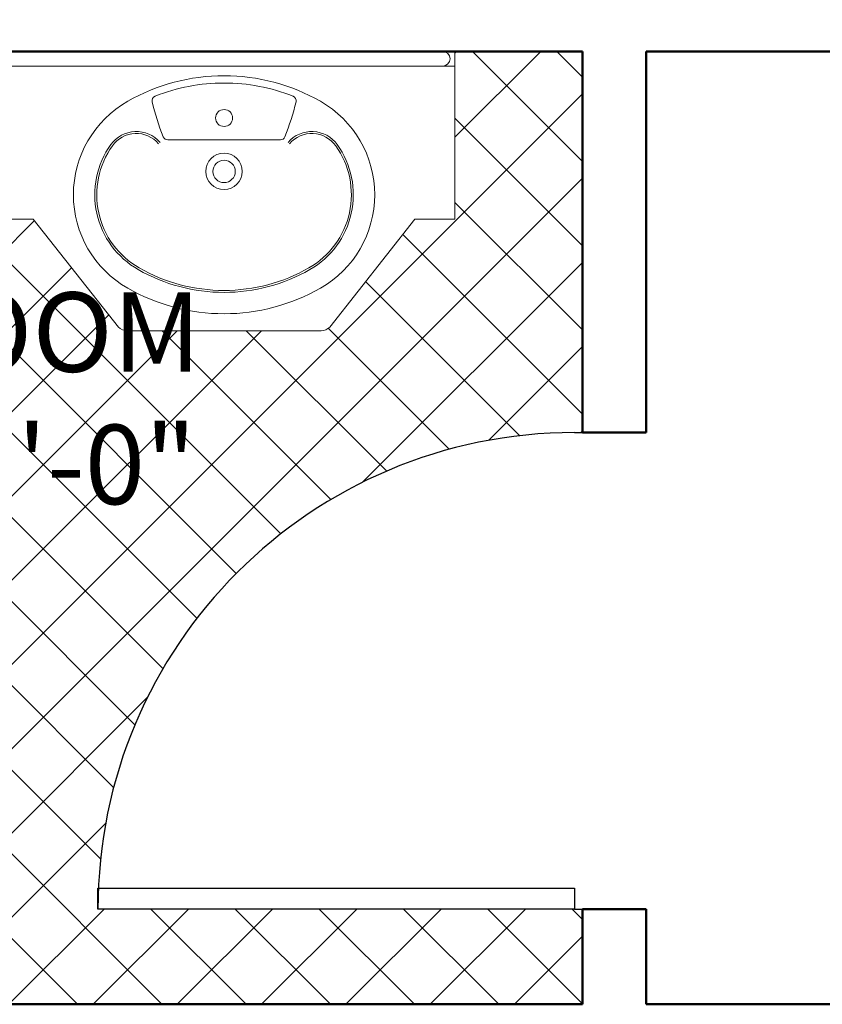
# Model space of a CAD drawing. Units: inches. Extents: x -466983 to 1020, y 324 to 318697.
# Tile 5 of 97: x 504 to 555, y 567 to 629. Entities that reach past the tile are written whole.
import ezdxf

# ---------------------------------------------------------------- set-up
doc = ezdxf.new("R2010")
doc.units = ezdxf.units.IN
doc.header["$MEASUREMENT"] = 0
for name, color, linetype, lineweight in [('A-AREA-IDEN', 7, 'Continuous', 25), ('A-DOOR', 3, 'Continuous', 25), ('A-FLOR-FIXT', 9, 'Continuous', 18), ('A-FLOR-PATT', 252, 'Continuous', 13), ('A-WALL', 7, 'Continuous', 50)]:
    doc.layers.add(name, color=color, linetype=linetype, lineweight=lineweight)
doc.styles.get("Standard").update_dxf_attribs({"font": 'arial.ttf'})

# ---------------------------------------------------------------- blocks, each defined once
blk = doc.blocks.new('*U33')
for p, q in [((0, 0), (-1e-16, -5.999999999999999)), ((40, -6e-16), (40, -6))]:
    blk.add_line(p, q)
blk.add_lwpolyline([(0, 0), (5.6e-15, 40), (1.750000000000007, 40), (1.749999999999998, -7e-16)], close=True)
blk.add_arc((0, 0), 40, 0, 90)
blk = doc.blocks.new('B3')
for p, q in [((-450, 0), (-455.7402514854766, -1.1418070123309)), ((450, 0), (455.7402514854766, -1.1418070123309)), ((-463.8581929876745, -9.25974851452338), (-465, -15)), ((-465, -15), (-463.8581929876745, -20.74025148547662)), ((-460.6066017178018, -4.393398282201815), (-463.8581929876745, -9.25974851452338)), ((-455.7402514854766, -1.1418070123309), (-460.6066017178018, -4.393398282201815)), ((455.7402514854766, -1.1418070123309), (460.6066017177945, -4.393398282201815)), ((460.6066017177945, -4.393398282201815), (463.8581929876672, -9.25974851452338)), ((463.8581929876672, -9.25974851452338), (465, -15)), ((465, -15), (463.8581929876672, -20.74025148547662)), ((475, -30), (-475, -30)), ((-463.8581929876745, -20.74025148547662), (-460.6066017178018, -25.60660171779819)), ((-460.6066017178018, -25.60660171779819), (-455.7402514854766, -28.8581929876691)), ((-455.7402514854766, -28.8581929876691), (-450, -30)), ((455.7402514854766, -28.8581929876691), (450, -30)), ((460.6066017177945, -25.60660171779819), (455.7402514854766, -28.8581929876691)), ((463.8581929876672, -20.74025148547662), (460.6066017177945, -25.60660171779819)), ((2.91038e-11, -182.0000000000054), (-115.8117069986983, -182.0000000000054)), ((2.91038e-11, -182.0000000000054), (115.8117069987565, -182.0000000000054))]:
    blk.add_line(p, q)
blk.add_lwpolyline([(199.4833683843535, -575, 0.2017697719241106), (217.3542190239823, -567.482353886593), (392.5, -345), (435, -345), (475, -345), (475, 0), (-475, 0), (-475, -345), (-435, -345), (-392.5, -345), (-217.3542190239896, -567.482353886593, 0.2017697719241107), (-199.4833683843608, -575)], format="xyb", close=True)
for centre, radius, start, end in [((5.09317e-11, -450.0000000000327), 400.0000000000322, 90, 119.7172288959075), ((0, -450.0000000000327), 400.0000000000319, 60.28277110409252, 90), ((2.91038e-11, -450.0000000000055), 385, 90, 111.6513567404431), ((2.91038e-11, -450.0000000000055), 385, 68.34864325955687, 90), ((-138.3591766736499, -101.4576952073475), 10, 111.6513567404431, 193.3915177581575), ((138.3591766737008, -101.4576952073475), 10, 346.6084822418425, 68.34864325955687), ((-88.47222222221171, -295.0000000000055), 221.527777777762, 119.7172288959075, 240.2827711040925), ((338.3178096717893, 12.0282100348104), 500, 193.3915177581575, 202.0594091764406), ((2.91038e-11, -136.9999999999891), 17.5, 90, 270), ((2.91038e-11, -136.9999999999891), 17.5, 270, 90), ((-338.3178096717383, 12.0282100348104), 500, 337.9405908235594, 346.6084822418425), ((88.47222222225537, -294.9999999999964), 221.527777777762, 299.7172288959074, 60.28277110409252), ((-180.5137974189128, -229.2550553338115), 64.41699441097052, 40.71477974361456, 144.4619255202982), ((-180.5137974189128, -229.2550553338115), 60.41699441097051, 40.71477974361456, 144.4619255202982), ((-115.8117069986983, -172.0000000000145), 10, 202.0594091764406, 270), ((115.8117069987565, -172.0000000000145), 10, 270, 337.9405908235594), ((180.5137974189638, -229.2550553338115), 64.41699441097052, 35.53807447970174, 139.2852202563854), ((180.5137974189638, -229.2550553338115), 60.41699441097051, 35.53807447970174, 139.2852202563854), ((-88.47222222221171, -295.0000000000055), 177.5277777777778, 144.4619255202982, 240.2827711040925), ((-88.47222222221171, -295.0000000000055), 173.5277777777778, 144.4619255202982, 240.2827711040925), ((88.47222222223354, -295.0000000000055), 173.5277777777778, 299.7172288959074, 35.53807447970174), ((88.47222222223354, -295.0000000000055), 177.5277777777778, 299.7172288959074, 35.53807447970174), ((2.91038e-11, -247.0000000000037), 37.5, 90, 270), ((2.91038e-11, -247.0000000000037), 37.5, 270, 90), ((2.91038e-11, -247.0000000000037), 23, 90, 270), ((2.91038e-11, -247.0000000000037), 23, 270, 90), ((2.91038e-11, -140.0000000000036), 352, 240.2827711040925, 270), ((2.91038e-11, -140.0000000000036), 352, 270, 299.7172288959074), ((2.91038e-11, -140.0000000000036), 356, 240.2827711040925, 270), ((2.91038e-11, -140.0000000000036), 356, 270, 299.7172288959074), ((5.09317e-11, -139.9999999999781), 400.0000000000309, 240.2827711040925, 270), ((-1.45519e-11, -140.0000000000309), 399.9999999999781, 270, 299.7172288959074)]:
    blk.add_arc(centre, radius, start, end)

msp = doc.modelspace()

# ---------------------------------------------------------------- hatches: boundary and pattern name
at = {"layer": 'A-FLOR-PATT', "transparency": 33554572}
h = msp.add_hatch(dxfattribs=at)
h.set_pattern_fill('ANSI37', color=256, scale=30)
h.set_pattern_definition([(45, (-1212.413693079869, -290.0350025265127), (-2.651650429449553, 2.651650429449553), []), (135, (-1212.413693079869, -290.0350025265127), (-2.651650429449553, -2.651650429449552), [])])
h.paths.add_polyline_path([(901.805677520904, 1075.937732818422), (900.6144036774049, 1075.937732818422), (900.6144036774049, 1065.385628316983), (899.390971271441, 1065.385628316983), (898.0910743401043, 1065.385628316983), (892.8355944880973, 1058.709752245277, -0.2583770168556315), (892.18750428989, 1058.350891982691), (879.9847834232776, 1058.350891982691, -0.2017697719240963), (879.438188978411, 1058.580825279484), (874.0812133730635, 1065.385628316983), (872.7813164417267, 1065.385628316983), (871.5578840357629, 1065.385628316983), (871.5578840357629, 1075.937732818422), (813.8056775209042, 1075.937732818422), (813.8056775209042, 1044.792233318721), (832.3947444543938, 1044.792233318721, -0.3947951267487684), (848.6601780212009, 1028.535584015862), (848.6601780212009, 1009.937732818421), (901.805677520904, 1009.937732818421), (901.805677520904, 1015.937732818421), (901.3056775209042, 1015.937732818421), (871.3056775209039, 1015.937732818421), (871.3056775209039, 1017.250232818421), (871.3344022102003, 1017.250232818421, -0.4014527144963572), (901.3056775209042, 1045.937732818421), (901.805677520904, 1045.937732818421)])
edge = h.paths.add_edge_path(flags=16)
edge.add_line((847.7730719745084, 1068.948588737025), (847.7730719745069, 1073.708823774771))
edge.add_arc((849.2268986539951, 1073.708823774771), 1.453826679487974, 90, 180, ccw=False)
edge.add_line((849.2268986539951, 1075.162650454259), (864.4920787886183, 1075.162650454259))
edge.add_arc((864.4920787886213, 1073.708823774771), 1.453826679487974, 0, 90.00000000012102, ccw=False)
edge.add_line((865.9459054681093, 1073.708823774771), (865.9459054681081, 1069.00351244647))
edge.add_arc((832.6447385074767, 1068.976050591752), 33.30117828385809, -20.61233806670998, 0.04724903539101888, ccw=False)
edge.add_ellipse((856.8594887213083, 1058.479989307073), major_axis=(-2.091e-13, 10.21313242340307), ratio=0.6859192225533502, start_angle=100.00884331843292, end_angle=259.9911566815624, ccw=False)
edge.add_arc((881.0742389351396, 1068.976050591752), 33.30117828385809, 180.0472490354062, 200.6123380667097, ccw=False)
h.paths.add_polyline_path([(853.145578187156, 1066.481532374271), (853.145578187156, 1066.453444752512), (853.1463399851561, 1066.453444752512, 0.4331071439582673), (852.9166149812349, 1066.684892837266), (852.9166149812349, 1066.453444752512), (853.145578187156, 1066.453444752512), (853.145578187156, 1066.481532374489), (853.088019486549, 1066.612171966583, 0.6979386910037918), (852.699540939094, 1066.453444752512), (852.7003027371272, 1066.453444752512), (852.7003027371272, 1066.481532374489), (852.9166149812349, 1067.001204630995), (852.9166149812349, 1066.684892837266, -0.3962543063594317)], flags=0)
h.paths.add_polyline_path([(861.0186747055222, 1066.481532374271), (861.0186747055222, 1066.453444752512), (861.0194365035225, 1066.453444752512, 0.4164039232557909), (860.8023624614146, 1066.684892837265), (860.8023624614146, 1066.453444752512), (861.0186747055222, 1066.453444752512), (861.0186747055222, 1066.481532374489), (860.9671752720659, 1066.605255499379, 0.7133437187663149), (860.5726374574602, 1066.453444752512), (860.5733992554934, 1066.453444752512), (860.5733992554934, 1066.481532374489), (860.8023624614146, 1067.001204630995), (860.8023624614146, 1066.684892837265, -0.3799725304814568)], flags=0)
edge = h.paths.add_edge_path(flags=0)
edge.add_spline(control_points=[(861.1298377106021, 1065.785468371534), (861.4660965533383, 1065.247811229462), (861.613385559155, 1065.016139861057), (861.9832837951076, 1064.373617117607), (862.1924105327118, 1063.944313665492), (862.5613774174725, 1063.039129539609), (862.7212131906668, 1062.56326642291), (862.9865156700853, 1061.578122280975), (863.0919804897928, 1061.068856600952), (863.2452407883674, 1060.031049745086), (863.293035446714, 1059.502522766744), (863.3294736797056, 1058.440879580113), (863.3181170778639, 1057.907777155726), (863.2366033468288, 1056.85179603536), (863.1664466211855, 1056.328931215311), (862.9695120306455, 1055.307951977375), (862.8427353108815, 1054.809852090196), (862.5365466723708, 1053.852219447362), (862.3571373353129, 1053.392702749349), (861.9514237071658, 1052.524888245794), (861.7251255454219, 1052.116609101398), (861.2330086320977, 1051.362239687588), (860.9672044472572, 1051.016170456457), (860.4047960485765, 1050.394909316517), (860.1082220871676, 1050.119734477926), (859.493696255806, 1049.64606200509), (859.1757900615103, 1049.447558762665), (858.5275631429041, 1049.129883644436), (858.197273503909, 1049.010664382187), (857.5314773710529, 1048.851811036626), (857.1959384637446, 1048.812116564677), (856.5249326641573, 1048.811967422545), (856.1893892160524, 1048.851512676201), (855.5235728169741, 1049.010066967686), (855.1932673158994, 1049.129136347874), (854.5449932971788, 1049.446513839261), (854.2270557868354, 1049.644869411481), (853.6124495619564, 1050.118254324803), (853.3158265363004, 1050.393289340464), (852.7533025914207, 1051.014284587242), (852.487431959371, 1051.360227769297), (851.9951668313728, 1052.114363776776), (851.7687869247744, 1052.522535562859), (851.3628973914427, 1053.390157753425), (851.1833939042357, 1053.849589492002), (850.8770077813263, 1054.807077270704), (850.7501277313783, 1055.30511724975), (850.5529806633081, 1056.326003473117), (850.4827147921034, 1056.848835185142), (850.4009803807432, 1057.904777820697), (850.3895122452288, 1058.437874867502), (850.425728471152, 1059.499535178563), (850.4734126571939, 1060.02808465918), (850.6264565107679, 1061.065963770327), (850.7318153592672, 1061.575279204679), (850.9969137893603, 1062.560548677974), (851.1566514873134, 1063.036487374614), (851.525433403113, 1063.94184619004), (851.7344732542367, 1064.371248757046), (852.1056260411488, 1065.016350037675), (852.2544071072941, 1065.250281998093), (852.608154630964, 1065.733465727338)], knot_values=[3.915332106759953, 3.915332106759953, 3.915332106759953, 3.915332106759953, 4.013467662305501, 4.013467662305501, 4.175531746215815, 4.175531746215815, 4.337595830126129, 4.337595830126129, 4.499659914036444, 4.499659914036444, 4.661723997946757, 4.661723997946757, 4.82378808185707, 4.82378808185707, 4.985852165767384, 4.985852165767384, 5.147916249677697, 5.147916249677697, 5.30998033358801, 5.30998033358801, 5.472044417498324, 5.472044417498324, 5.634108501408637, 5.634108501408637, 5.79617258531895, 5.79617258531895, 5.958236669229264, 5.958236669229264, 6.120300753139577, 6.120300753139577, 6.282364837049891, 6.282364837049891, 6.444428920960204, 6.444428920960204, 6.606493004870517, 6.606493004870517, 6.768557088780831, 6.768557088780831, 6.930621172691144, 6.930621172691144, 7.092685256601457, 7.092685256601457, 7.254749340511771, 7.254749340511771, 7.416813424422084, 7.416813424422084, 7.578877508332397, 7.578877508332397, 7.740941592242711, 7.740941592242711, 7.903005676153024, 7.903005676153024, 8.065069760063338, 8.065069760063338, 8.22713384397365, 8.22713384397365, 8.389197927883965, 8.389197927883965, 8.551262011794279, 8.551262011794279, 8.650370494357087, 8.650370494357087, 8.650370494357087, 8.650370494357087], degree=3, periodic=0)
edge.add_line((852.6421178657537, 1065.785468371534), (861.1298377106024, 1065.785468371534))
edge = h.paths.add_edge_path(flags=0)
edge.add_ellipse((856.8495804607978, 1057.743205248224), major_axis=(-3.1e-13, 7.792134415209829), ratio=0.6878610933899516, start_angle=0, end_angle=360)
h.paths.add_polyline_path([(848.8634419841151, 1069.389059844444), (848.863441984139, 1073.960453158315, -0.4142135623709757), (849.9538119937549, 1075.050823167924), (863.765165448898, 1075.050823167924, -0.4142135623721942), (864.8555354585106, 1073.960453158308), (864.8555354584933, 1069.389059844444, -0.3889362887010341), (864.5236837164459, 1069.026979909221, -0.0435607626104464), (849.19529372618, 1069.02697990933, -0.3889362886276668)], flags=0)
h.paths.add_polyline_path([(853.1006153779753, 1068.112209480768, -1), (852.677499999749, 1068.112209480768, -1)], flags=0)
edge = h.paths.add_edge_path(flags=0)
edge.add_ellipse((856.8594887213083, 1057.33782914961), major_axis=(7.74e-14, 2.20702192546696), ratio=0.6571642650458812, start_angle=0, end_angle=360)
h.paths.add_polyline_path([(861.0414774428674, 1068.112209480768, -1), (860.6183620646412, 1068.112209480768, -1)], flags=0)
edge = h.paths.add_edge_path()
edge.add_line((573.9536545579417, 1057.341203598636), (573.9536545579417, 1075.937732818422))
edge.add_line((573.9536545579417, 1075.937732818422), (558.7307922536265, 1075.937732818422))
edge.add_line((558.7307922536265, 1075.937732818422), (558.7307922536265, 1065.385628316983))
edge.add_line((558.7307922536265, 1065.385628316983), (557.5073598476627, 1065.385628316983))
edge.add_line((557.5073598476627, 1065.385628316983), (556.207462916326, 1065.385628316983))
edge.add_line((556.207462916326, 1065.385628316983), (550.9519830643189, 1058.709752245277))
edge.add_arc((550.3038928661116, 1059.115537236419), 0.7646452537275144, 270, 327.94831933647396, ccw=False)
edge.add_line((550.3038928661116, 1058.350891982691), (538.1011719994992, 1058.350891982691))
edge.add_arc((538.1011719994992, 1059.115537236419), 0.7646452537275137, 224.3704013916024, 270, ccw=False)
edge.add_line((537.5545775546327, 1058.580825279484), (532.1976019492852, 1065.385628316983))
edge.add_line((532.1976019492852, 1065.385628316983), (530.8977050179485, 1065.385628316983))
edge.add_line((530.8977050179485, 1065.385628316983), (529.6742726119846, 1065.385628316983))
edge.add_line((529.6742726119846, 1065.385628316983), (529.6742726119846, 1075.937732818422))
edge.add_line((529.6742726119846, 1075.937732818422), (520.8056775209042, 1075.937732818422))
edge.add_line((520.8056775209042, 1075.937732818422), (520.8056775209042, 1045.937732818422))
edge.add_line((520.8056775209042, 1045.937732818422), (521.3056775209044, 1045.937732818422))
edge.add_arc((521.3056775209042, 1015.937732818422), 30.00000000000023, 2.507490703587223, 89.99999999999977, ccw=False)
edge.add_line((551.2769528316082, 1017.250232818422), (551.3056775209045, 1017.250232818422))
edge.add_line((551.3056775209045, 1017.250232818422), (551.3056775209045, 1015.937732818422))
edge.add_line((551.3056775209045, 1015.937732818422), (520.8056775209042, 1015.937732818422))
edge.add_line((520.8056775209042, 1015.937732818422), (520.8056775209042, 1009.937732818421))
edge.add_line((520.8056775209042, 1009.937732818421), (559.1912990237018, 1010.402158339383))
edge.add_arc((559.1912990237018, 1011.855985018871), 1.453826679487974, 180, 270, ccw=False)
edge.add_line((557.7374723442138, 1011.855985018871), (557.7374723442151, 1016.561296347171))
edge.add_arc((591.0386393048469, 1016.58875820189), 33.3011782838587, 159.3876619332891, 180.0472490353913, ccw=False)
edge.add_ellipse((566.8238890910148, 1027.084819486569), major_axis=(-3.171e-13, 10.21313242340307), ratio=0.6859192225533445, start_angle=280.00884331843395, end_angle=439.99115668156304, ccw=False)
edge.add_arc((542.6091388771833, 1016.58875820189), 33.3011782838584, 0.04724903544490644, 20.612338066710322, ccw=False)
edge.add_line((575.9103058378148, 1016.61622005664), (575.910305837816, 1011.855985018871))
edge.add_arc((574.4564791583282, 1011.855985018871), 1.453826679487974, -90, 0, ccw=False)
edge.add_line((574.4564791583282, 1010.402158339383), (608.8056775209044, 1009.937732818421))
edge.add_line((608.8056775209044, 1009.937732818421), (608.8056775209044, 1041.08570985546))
edge.add_line((608.8056775209044, 1041.08570985546), (590.2179319406538, 1041.08570985546))
edge.add_arc((590.7750219589672, 1057.907380652626), 16.83089295601249, 181.9277454211679, 268.1032059320871, ccw=False)
edge = h.paths.add_edge_path()
edge.add_ellipse((494.2443328575609, 583.6203939656394), major_axis=(-2.099e-13, 10.21313242340307), ratio=0.6859192225533391, start_angle=280.0088433184392, end_angle=439.99115668155895, ccw=False)
edge.add_arc((470.0295826437295, 573.1243326809605), 33.30117828385828, 0.047249035653180727, 20.612338066711573, ccw=False)
edge.add_line((503.3307496043607, 573.1517945358311), (503.3307496043621, 568.3915594979414))
edge.add_arc((501.8769229248741, 568.3915594979414), 1.453826679487974, -90, 0, ccw=False)
edge.add_line((501.8769229248741, 566.9377328184536), (539.8056775209043, 566.9377328184218))
edge.add_line((539.8056775209043, 566.9377328184218), (539.8056775209043, 572.9377328184218))
edge.add_line((539.8056775209043, 572.9377328184218), (539.3056775209043, 572.9377328184218))
edge.add_line((539.3056775209043, 572.9377328184218), (509.3056775209042, 572.9377328184218))
edge.add_line((509.3056775209042, 572.9377328184218), (509.3056775209042, 574.2502328184218))
edge.add_line((509.3056775209042, 574.2502328184218), (509.3344022102004, 574.2502328184218))
edge.add_arc((539.3056775209043, 572.9377328184218), 30.00000000000003, 90, 177.4925092964128, ccw=False)
edge.add_line((539.3056775209043, 602.9377328184218), (539.8056775209043, 602.9377328184218))
edge.add_line((539.8056775209043, 602.9377328184218), (539.8056775209043, 626.9377328184219))
edge.add_line((539.8056775209043, 626.9377328184219), (531.7718318056131, 626.9377328184219))
edge.add_line((531.7718318056131, 626.9377328184219), (531.7718318056131, 616.3856283169836))
edge.add_line((531.7718318056131, 616.3856283169836), (530.5483993996492, 616.3856283169836))
edge.add_line((530.5483993996492, 616.3856283169836), (529.2485024683125, 616.3856283169836))
edge.add_line((529.2485024683125, 616.3856283169836), (523.7105154427977, 609.3508919826913))
edge.add_line((523.7105154427977, 609.3508919826913), (510.7766285267865, 609.3508919826913))
edge.add_line((510.7766285267865, 609.3508919826913), (505.2386415012717, 616.3856283169835))
edge.add_line((505.2386415012717, 616.3856283169835), (503.9387445699351, 616.3856283169836))
edge.add_line((503.9387445699351, 616.3856283169836), (502.7153121639711, 616.3856283169836))
edge.add_line((502.7153121639711, 616.3856283169836), (502.7153121639712, 626.9377328184219))
edge.add_line((502.7153121639712, 626.9377328184219), (481.698294634846, 626.937732818422))
edge.add_line((481.698294634846, 626.937732818422), (481.6982946348461, 610.9950036909872))
edge.add_arc((467.2703297247223, 611.4728203914133), 14.43587476556121, 271.9277454211847, 358.103205932099, ccw=False)
edge.add_line((467.7559403853078, 597.0451157044822), (451.8056775209041, 597.0451157044822))
edge.add_line((451.8056775209041, 597.0451157044822), (451.8056775209041, 584.4035114605515))
edge.add_line((451.8056775209041, 584.4035114605515), (451.8056775209043, 566.9377328184218))
edge.add_line((451.8056775209043, 566.9377328184218), (486.6117427902477, 566.9377328184536))
edge.add_arc((486.6117427902477, 568.3915594979414), 1.453826679487974, 180, 270, ccw=False)
edge.add_line((485.1579161107598, 568.3915594979414), (485.157916110761, 573.0968708261933))
edge.add_arc((518.4590830713927, 573.1243326809608), 33.3011782838585, 159.387661933289, 180.0472490354759, ccw=False)
h.paths.add_polyline_path([(836.2608886421394, 1020.732838196592), (879.8898108795202, 1020.732838196592), (879.8898108795202, 1039.390182443977), (836.2608886421394, 1039.390182443977)], flags=25)
h.paths.add_polyline_path([(549.9851009445293, 1036.749159167106), (593.6140231819099, 1036.749159167106), (593.6140231819099, 1055.406503414491), (549.9851009445293, 1055.406503414491)], flags=24)
h.paths.add_polyline_path([(475.1230325221868, 595.5958681380167), (518.7519547595675, 595.5958681380167), (518.7519547595675, 614.2532123854019), (475.1230325221868, 614.2532123854019)], flags=24)

# ---------------------------------------------------------------- linework, layer by layer
at = {"layer": 'A-WALL'}
for p, q in [((539.8056775209043, 626.9377328184219), (451.8056775209042, 626.9377328184219)), ((539.8056775209043, 602.9377328184219), (539.8056775209043, 626.9377328184219)), ((612.8056775209044, 626.9377328184219), (543.805677520904, 626.9377328184218)), ((543.805677520904, 602.9377328184219), (543.805677520904, 626.9377328184218)), ((543.8056775209044, 602.9377328184218), (539.8056775209043, 602.9377328184218)), ((539.8056775209043, 566.9377328184218), (539.8056775209043, 572.9377328184218)), ((543.8056775209044, 572.9377328184218), (539.8056775209043, 572.9377328184218)), ((543.8056775209043, 566.9377328184218), (543.8056775209043, 572.9377328184218)), ((539.8056775209043, 566.9377328184218), (451.8056775209041, 566.9377328184218)), ((566.8056775209044, 566.9377328184218), (543.8056775209043, 566.9377328184218))]:
    msp.add_line(p, q, dxfattribs=at)

# ---------------------------------------------------------------- block references
at = {"layer": 'A-DOOR', "xscale": 0.7500000000000007, "yscale": 0.7500000000000007, "zscale": 0.7500000000000007, "rotation": 90}
msp.add_blockref('*U33', (539.3056775209043, 572.9377328184218), dxfattribs=at)
at = {"layer": 'A-FLOR-FIXT', "xscale": 0.0305858101490967, "yscale": 0.0305858101490967, "zscale": 0.0305858101490967}
msp.add_blockref('B3', (517.2435719847921, 626.9377328184219), dxfattribs=at)

# ---------------------------------------------------------------- texts
at = {"layer": 'A-AREA-IDEN', "insert": (461.9844353108056, 611.7651496296038), "char_height": 5, "attachment_point": 1}
msp.add_mtext_dynamic_manual_height_columns('\\pxqc;{\\fArial|b1|i0|c0|p34;BATHROOM\\P7\'-4" X 5\'-0"}', width=69.92316986614605, gutter_width=1, heights=[0], dxfattribs=at)

doc.saveas('drawing.dxf')
